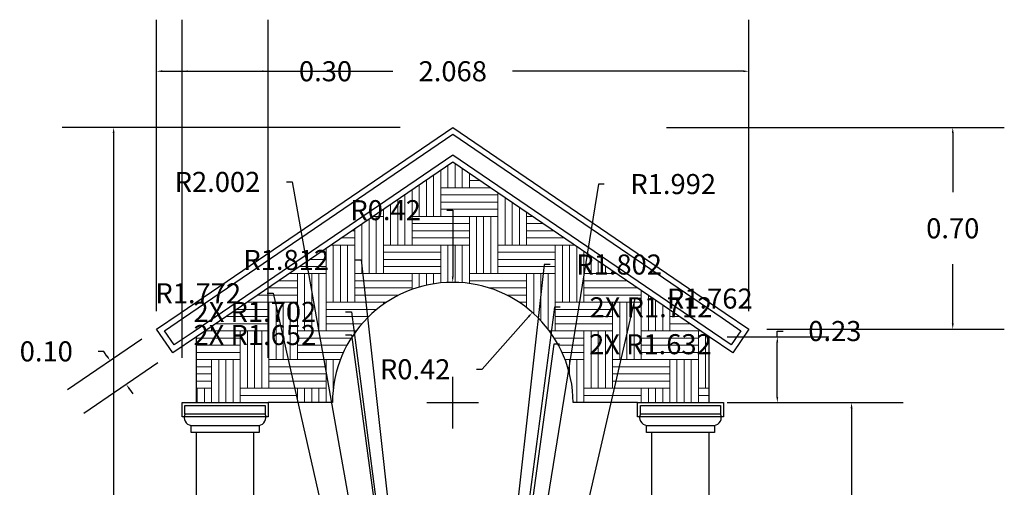
# Model space of a CAD drawing. Units: metres. Extents: x 10.71 to 14.27, y 9.22 to 13.79.
# Tile 2 of 2: x 10.83 to 14.27, y 12.15 to 13.79. Entities that reach past the tile are written whole.
import ezdxf

# ---------------------------------------------------------------- set-up
doc = ezdxf.new("R2010")
doc.units = ezdxf.units.M
doc.header["$MEASUREMENT"] = 0
for name, color, linetype, lineweight in [('A-ANNO-DIMS', 2, 'Continuous', 18), ('A-COLS', 7, 'Continuous', 30), ('A-ROOF', 7, 'Continuous', 30), ('A-ROOF-PATT', 252, 'Continuous', 13)]:
    doc.layers.add(name, color=color, linetype=linetype, lineweight=lineweight)
doc.styles.get("Standard").update_dxf_attribs({"font": 'arial.ttf'})
doc.dimstyles.get("Standard").update_dxf_attribs({"dimtxt": 0.07, "dimasz": 0.02, "dimexe": 0.18, "dimexo": 0.0625, "dimgap": 0.09, "dimtad": 0, "dimtih": 1, "dimtoh": 1, "dimzin": 0, "dimdsep": 46, "dimtxsty": 'Standard', "dimcen": 0.09, "dimadec": 0, "dimazin": 0, "dimtfac": 1, "dimtofl": 0, "dimtmove": 0, "dimatfit": 3, "dimfxl": 1, "dimfxlon": 1, "dimtolj": 1, "dimtzin": 0, "dimarcsym": 0})

# ---------------------------------------------------------------- blocks, each defined once
blk = doc.blocks.new('*D4')
at = {"layer": 'A-ANNO-DIMS', "color": 0, "lineweight": -2, "transparency": 16777216}
for p, q in [((12.1582, 13.4108), (10.9782, 13.4108)), ((11.1582, 13.3908), (11.1582, 11.7313)), ((11.1582, 9.8203), (11.1582, 11.4798)), ((11.1582, 9.8003), (10.9782, 9.8003))]:
    blk.add_line(p, q, dxfattribs=at)
at = {"layer": 'A-ANNO-DIMS', "color": 0, "transparency": 16777216}
for points in [[(11.1548, 13.3908), (11.1615, 13.3908), (11.1582, 13.4108)], [(11.1548, 9.8203), (11.1615, 9.8203), (11.1582, 9.8003)]]:
    blk.add_solid(points, dxfattribs=at)
at = {"layer": 'Defpoints', "color": 0, "transparency": 16777216}
for p in [(11.1582, 13.4108), (12.3422, 13.4108), (11.1842, 9.8003)]:
    blk.add_point(p, dxfattribs=at)
at = {"layer": 'A-ANNO-DIMS', "color": 0, "transparency": 16777216, "insert": (11.1582, 11.6055), "char_height": 0.07, "attachment_point": 5}
blk.add_mtext('\\A1;3.61', dxfattribs=at)
blk = doc.blocks.new('*D5')
at = {"layer": 'A-ANNO-DIMS', "color": 0, "lineweight": -2, "transparency": 16777216}
for p, q in [((13.4753, 12.6798), (13.4753, 12.6998)), ((13.4753, 12.6998), (13.4953, 12.6998)), ((13.2997, 12.6798), (13.6553, 12.6798)), ((13.4753, 12.4698), (13.4753, 12.6598)), ((13.2997, 12.4498), (13.6553, 12.4498))]:
    blk.add_line(p, q, dxfattribs=at)
at = {"layer": 'A-ANNO-DIMS', "color": 0, "transparency": 16777216}
for points in [[(13.472, 12.6598), (13.4786, 12.6598), (13.4753, 12.6798)], [(13.472, 12.4698), (13.4786, 12.4698), (13.4753, 12.4498)]]:
    blk.add_solid(points, dxfattribs=at)
at = {"layer": 'Defpoints', "color": 0, "transparency": 16777216}
for p in [(13.2372, 12.6798), (13.4753, 12.6798), (13.2372, 12.4498)]:
    blk.add_point(p, dxfattribs=at)
at = {"layer": 'A-ANNO-DIMS', "color": 0, "transparency": 16777216, "insert": (13.6762, 12.6998), "char_height": 0.07, "attachment_point": 5}
blk.add_mtext('\\A1;0.23', dxfattribs=at)
blk = doc.blocks.new('*D9')
at = {"layer": 'A-ANNO-DIMS', "color": 0, "lineweight": -2, "transparency": 16777216}
for p, q in [((12.445, 12.5663), (12.6068, 12.7498)), ((12.425, 12.5663), (12.445, 12.5663))]:
    blk.add_line(p, q, dxfattribs=at)
at = {"layer": 'A-ANNO-DIMS', "color": 0, "transparency": 16777216}
blk.add_solid([(12.6043, 12.752), (12.6093, 12.7476), (12.62, 12.7648)], dxfattribs=at)
at = {"layer": 'Defpoints', "color": 0, "transparency": 16777216}
for p in [(12.62, 12.7648), (12.3422, 12.4498)]:
    blk.add_point(p, dxfattribs=at)
at = {"layer": 'A-ANNO-DIMS', "color": 0, "transparency": 16777216, "insert": (12.2109, 12.5663), "char_height": 0.07, "attachment_point": 5}
blk.add_mtext('\\A1;R0.42', dxfattribs=at)
blk = doc.blocks.new('COL-ENTRANCE-CLASSICAL')
for p, q in [((0.1002, 1.975), (0.1002, 2.545)), ((0.3002, 1.975), (0.3002, 2.545)), ((0.1002, 0.1003), (0.1002, 1.8703)), ((0.3002, 0.1003), (0.3002, 1.8703)), ((0.1002, 0.1003), (0.3002, 0.1003))]:
    blk.add_line(p, q)
for points in [[(0.0502, 2.6498), (0.3502, 2.6498), (0.3502, 2.5998), (0.0502, 2.5998)], [(0.0602, 2.6398), (0.3402, 2.6398), (0.3402, 2.6098), (0.0602, 2.6098)], [(0.0816, 2.5705), (0.319, 2.5705), (0.319, 2.545), (0.0816, 2.545)], [(0.0502, 1.975), (0.3502, 1.975), (0.3502, 1.925), (0.0502, 1.925)], [(0.0602, 1.965), (0.3402, 1.965), (0.3402, 1.935), (0.0602, 1.935)], [(0.0816, 1.8957), (0.319, 1.8957), (0.319, 1.8703), (0.0816, 1.8703)], [(0.0502, 0.1003), (0.3502, 0.1003), (0.3502, 0.0503), (0.0502, 0.0503)], [(0.0602, 0.0903), (0.3402, 0.0903), (0.3402, 0.0603), (0.0602, 0.0603)], [(0.0002, 0.0503), (0.4002, 0.0503), (0.4002, 0.0003), (0.0002, 0.0003)], [(0.0102, 0.0403), (0.3902, 0.0403), (0.3902, 0.0103), (0.0102, 0.0103)]]:
    blk.add_lwpolyline(points, close=True)
for centre, radius, start, end in [((0.0856, 2.5981), 0.0279, 155.2605, 261.7776), ((0.3152, 2.5979), 0.0277, 277.9826, 25.4449), ((0.0856, 1.9233), 0.0279, 155.2605, 261.7776), ((0.3152, 1.9231), 0.0277, 277.9826, 25.4449)]:
    blk.add_arc(centre, radius, start, end)
blk = doc.blocks.new('*D15')
at = {"layer": 'A-ANNO-DIMS', "color": 0, "lineweight": -2, "transparency": 16777216}
for p, q in [((13.3997, 12.4498), (13.9146, 12.4498)), ((13.7346, 12.4298), (13.7346, 11.2512)), ((13.7346, 9.8203), (13.7346, 10.9988)), ((13.3997, 9.8003), (13.9146, 9.8003))]:
    blk.add_line(p, q, dxfattribs=at)
at = {"layer": 'A-ANNO-DIMS', "color": 0, "transparency": 16777216}
for points in [[(13.7313, 12.4298), (13.738, 12.4298), (13.7346, 12.4498)], [(13.7313, 9.8203), (13.738, 9.8203), (13.7346, 9.8003)]]:
    blk.add_solid(points, dxfattribs=at)
at = {"layer": 'Defpoints', "color": 0, "transparency": 16777216}
for p in [(13.3372, 12.4498), (13.7346, 12.4498), (13.3372, 9.8003)]:
    blk.add_point(p, dxfattribs=at)
at = {"layer": 'A-ANNO-DIMS', "color": 0, "transparency": 16777216, "insert": (13.7346, 11.125), "char_height": 0.07, "attachment_point": 5}
blk.add_mtext('\\A1;COLUMN 2.65 TYP.', dxfattribs=at)
blk = doc.blocks.new('*D19')
at = {"layer": 'A-ANNO-DIMS', "color": 0, "lineweight": -2, "transparency": 16777216}
for p, q in [((11.3082, 12.7686), (11.3082, 13.7868)), ((13.3762, 12.7686), (13.3762, 13.7868)), ((11.3283, 13.6068), (12.1334, 13.6068)), ((13.3562, 13.6068), (12.551, 13.6068))]:
    blk.add_line(p, q, dxfattribs=at)
at = {"layer": 'A-ANNO-DIMS', "color": 0, "transparency": 16777216}
for points in [[(11.3283, 13.6101), (11.3283, 13.6035), (11.3082, 13.6068)], [(13.3562, 13.6101), (13.3562, 13.6035), (13.3762, 13.6068)]]:
    blk.add_solid(points, dxfattribs=at)
at = {"layer": 'Defpoints', "color": 0, "transparency": 16777216}
for p in [(13.3762, 13.6068), (11.3082, 12.7061), (13.3762, 12.7061)]:
    blk.add_point(p, dxfattribs=at)
at = {"layer": 'A-ANNO-DIMS', "color": 0, "transparency": 16777216, "insert": (12.3422, 13.6068), "char_height": 0.07, "attachment_point": 5}
blk.add_mtext('\\A1;2.068', dxfattribs=at)
blk = doc.blocks.new('*D20')
at = {"layer": 'A-ANNO-DIMS', "color": 0, "lineweight": -2, "transparency": 16777216}
for p, q in [((13.0879, 13.4108), (14.2679, 13.4108)), ((14.0879, 13.3908), (14.0879, 13.1842)), ((14.0879, 12.7261), (14.0879, 12.9327)), ((13.4387, 12.7061), (14.2679, 12.7061))]:
    blk.add_line(p, q, dxfattribs=at)
at = {"layer": 'A-ANNO-DIMS', "color": 0, "transparency": 16777216}
for points in [[(14.0846, 13.3908), (14.0912, 13.3908), (14.0879, 13.4108)], [(14.0846, 12.7261), (14.0912, 12.7261), (14.0879, 12.7061)]]:
    blk.add_solid(points, dxfattribs=at)
at = {"layer": 'Defpoints', "color": 0, "transparency": 16777216}
for p in [(12.3422, 13.4108), (14.0879, 13.4108), (13.3762, 12.7061)]:
    blk.add_point(p, dxfattribs=at)
at = {"layer": 'A-ANNO-DIMS', "color": 0, "transparency": 16777216, "insert": (14.0879, 13.0584), "char_height": 0.07, "attachment_point": 5}
blk.add_mtext('\\A1;0.70', dxfattribs=at)
blk = doc.blocks.new('*D21')
at = {"layer": 'A-ANNO-DIMS', "color": 0, "lineweight": -2, "transparency": 16777216}
for p, q in [((11.2566, 12.6709), (10.9976, 12.4943)), ((11.1238, 12.6288), (11.1038, 12.6288)), ((11.135, 12.6122), (11.1238, 12.6288)), ((11.3129, 12.5883), (11.0539, 12.4117)), ((11.2139, 12.4965), (11.2251, 12.48))]:
    blk.add_line(p, q, dxfattribs=at)
at = {"layer": 'A-ANNO-DIMS', "color": 0, "transparency": 16777216}
for points in [[(11.1378, 12.6141), (11.1323, 12.6104), (11.1463, 12.5957)], [(11.2166, 12.4984), (11.2111, 12.4947), (11.2026, 12.5131)]]:
    blk.add_solid(points, dxfattribs=at)
at = {"layer": 'Defpoints', "color": 0, "transparency": 16777216}
for p in [(11.3082, 12.7061), (11.3646, 12.6235), (11.1463, 12.5957)]:
    blk.add_point(p, dxfattribs=at)
at = {"layer": 'A-ANNO-DIMS', "color": 0, "transparency": 16777216, "insert": (10.923, 12.6288), "char_height": 0.07, "attachment_point": 5}
blk.add_mtext('\\A1;0.10', dxfattribs=at)
blk = doc.blocks.new('*D24')
at = {"layer": 'A-ANNO-DIMS', "color": 0, "lineweight": -2, "transparency": 16777216}
for p, q in [((11.3972, 12.6068), (11.3972, 13.7868)), ((11.6972, 12.6068), (11.6972, 13.7868)), ((11.4172, 13.6068), (11.6772, 13.6068)), ((11.6972, 13.6068), (11.7172, 13.6068))]:
    blk.add_line(p, q, dxfattribs=at)
at = {"layer": 'A-ANNO-DIMS', "color": 0, "transparency": 16777216}
for points in [[(11.4172, 13.6101), (11.4172, 13.6035), (11.3972, 13.6068)], [(11.6772, 13.6101), (11.6772, 13.6035), (11.6972, 13.6068)]]:
    blk.add_solid(points, dxfattribs=at)
at = {"layer": 'Defpoints', "color": 0, "transparency": 16777216}
for p in [(11.6972, 13.6068), (11.3972, 11.775), (11.6972, 11.775)]:
    blk.add_point(p, dxfattribs=at)
at = {"layer": 'A-ANNO-DIMS', "color": 0, "transparency": 16777216, "insert": (11.898, 13.6068), "char_height": 0.07, "attachment_point": 5}
blk.add_mtext('\\A1;0.30', dxfattribs=at)
blk = doc.blocks.new('*D28')
at = {"layer": 'A-ANNO-DIMS', "color": 0, "lineweight": -2, "transparency": 16777216}
for p, q in [((11.762, 13.2204), (11.782, 13.2204)), ((11.782, 13.2204), (11.9886, 12.0574)), ((12.3422, 9.9765), (12.3422, 10.1565)), ((12.2522, 10.0665), (12.4322, 10.0665))]:
    blk.add_line(p, q, dxfattribs=at)
at = {"layer": 'A-ANNO-DIMS', "color": 0, "transparency": 16777216}
blk.add_solid([(11.9918, 12.058), (11.9853, 12.0568), (11.9921, 12.0377)], dxfattribs=at)
at = {"layer": 'Defpoints', "color": 0, "transparency": 16777216}
for p in [(11.9921, 12.0377), (12.3422, 10.0665)]:
    blk.add_point(p, dxfattribs=at)
at = {"layer": 'A-ANNO-DIMS', "color": 0, "transparency": 16777216, "insert": (11.5207, 13.2204), "char_height": 0.07, "attachment_point": 5}
blk.add_mtext('\\A1;R2.002', dxfattribs=at)
blk = doc.blocks.new('*D29')
at = {"layer": 'A-ANNO-DIMS', "color": 0, "lineweight": -2, "transparency": 16777216}
for p, q in [((12.8507, 13.2129), (12.6632, 12.0528)), ((12.8707, 13.2129), (12.8507, 13.2129)), ((12.3422, 9.9765), (12.3422, 10.1565)), ((12.2522, 10.0665), (12.4322, 10.0665))]:
    blk.add_line(p, q, dxfattribs=at)
at = {"layer": 'A-ANNO-DIMS', "color": 0, "transparency": 16777216}
blk.add_solid([(12.6599, 12.0533), (12.6665, 12.0522), (12.66, 12.033)], dxfattribs=at)
at = {"layer": 'Defpoints', "color": 0, "transparency": 16777216}
for p in [(12.66, 12.033), (12.3422, 10.0665)]:
    blk.add_point(p, dxfattribs=at)
at = {"layer": 'A-ANNO-DIMS', "color": 0, "transparency": 16777216, "insert": (13.1119, 13.2129), "char_height": 0.07, "attachment_point": 5}
blk.add_mtext('\\A1;R1.992', dxfattribs=at)
blk = doc.blocks.new('*D30')
at = {"layer": 'A-ANNO-DIMS', "color": 0, "lineweight": -2, "transparency": 16777216}
for p, q in [((12.002, 12.948), (12.022, 12.948)), ((12.022, 12.948), (12.1399, 11.8873)), ((12.3422, 9.9765), (12.3422, 10.1565)), ((12.2522, 10.0665), (12.4322, 10.0665))]:
    blk.add_line(p, q, dxfattribs=at)
at = {"layer": 'A-ANNO-DIMS', "color": 0, "transparency": 16777216}
blk.add_solid([(12.1432, 11.8877), (12.1365, 11.887), (12.1421, 11.8675)], dxfattribs=at)
at = {"layer": 'Defpoints', "color": 0, "transparency": 16777216}
for p in [(12.1421, 11.8675), (12.3422, 10.0665)]:
    blk.add_point(p, dxfattribs=at)
at = {"layer": 'A-ANNO-DIMS', "color": 0, "transparency": 16777216, "insert": (11.7607, 12.948), "char_height": 0.07, "attachment_point": 5}
blk.add_mtext('\\A1;R1.812', dxfattribs=at)
blk = doc.blocks.new('*D31')
at = {"layer": 'A-ANNO-DIMS', "color": 0, "lineweight": -2, "transparency": 16777216}
for p, q in [((12.6618, 12.932), (12.5442, 11.8773)), ((12.6818, 12.932), (12.6618, 12.932)), ((12.3422, 9.9765), (12.3422, 10.1565)), ((12.2522, 10.0665), (12.4322, 10.0665))]:
    blk.add_line(p, q, dxfattribs=at)
at = {"layer": 'A-ANNO-DIMS', "color": 0, "transparency": 16777216}
blk.add_solid([(12.5408, 11.8777), (12.5475, 11.8769), (12.5419, 11.8574)], dxfattribs=at)
at = {"layer": 'Defpoints', "color": 0, "transparency": 16777216}
for p in [(12.5419, 11.8574), (12.3422, 10.0665)]:
    blk.add_point(p, dxfattribs=at)
at = {"layer": 'A-ANNO-DIMS', "color": 0, "transparency": 16777216, "insert": (12.923, 12.932), "char_height": 0.07, "attachment_point": 5}
blk.add_mtext('\\A1;R1.802', dxfattribs=at)
blk = doc.blocks.new('*D32')
at = {"layer": 'A-ANNO-DIMS', "color": 0, "lineweight": -2, "transparency": 16777216}
for p, q in [((11.6948, 12.8315), (11.7148, 12.8315)), ((11.7148, 12.8315), (11.9457, 11.8141)), ((12.3422, 9.9765), (12.3422, 10.1565)), ((12.2522, 10.0665), (12.4322, 10.0665))]:
    blk.add_line(p, q, dxfattribs=at)
at = {"layer": 'A-ANNO-DIMS', "color": 0, "transparency": 16777216}
blk.add_solid([(11.9489, 11.8149), (11.9424, 11.8134), (11.9501, 11.7946)], dxfattribs=at)
at = {"layer": 'Defpoints', "color": 0, "transparency": 16777216}
for p in [(11.9501, 11.7946), (12.3422, 10.0665)]:
    blk.add_point(p, dxfattribs=at)
at = {"layer": 'A-ANNO-DIMS', "color": 0, "transparency": 16777216, "insert": (11.4536, 12.8315), "char_height": 0.07, "attachment_point": 5}
blk.add_mtext('\\A1;R1.772', dxfattribs=at)
blk = doc.blocks.new('*D33')
at = {"layer": 'A-ANNO-DIMS', "color": 0, "lineweight": -2, "transparency": 16777216}
for p, q in [((12.9783, 12.8131), (12.7443, 11.8026)), ((12.9983, 12.8131), (12.9783, 12.8131)), ((12.3422, 9.9765), (12.3422, 10.1565)), ((12.2522, 10.0665), (12.4322, 10.0665))]:
    blk.add_line(p, q, dxfattribs=at)
at = {"layer": 'A-ANNO-DIMS', "color": 0, "transparency": 16777216}
blk.add_solid([(12.7411, 11.8033), (12.7476, 11.8018), (12.7398, 11.7831)], dxfattribs=at)
at = {"layer": 'Defpoints', "color": 0, "transparency": 16777216}
for p in [(12.7398, 11.7831), (12.3422, 10.0665)]:
    blk.add_point(p, dxfattribs=at)
at = {"layer": 'A-ANNO-DIMS', "color": 0, "transparency": 16777216, "insert": (13.2396, 12.8131), "char_height": 0.07, "attachment_point": 5}
blk.add_mtext('\\A1;R1.762', dxfattribs=at)
blk = doc.blocks.new('*D34')
at = {"layer": 'A-ANNO-DIMS', "color": 0, "lineweight": -2, "transparency": 16777216}
for p, q in [((12.6971, 12.7827), (12.5666, 11.7839)), ((12.7171, 12.7827), (12.6971, 12.7827)), ((12.3422, 9.9765), (12.3422, 10.1565)), ((12.2522, 10.0665), (12.4322, 10.0665))]:
    blk.add_line(p, q, dxfattribs=at)
at = {"layer": 'A-ANNO-DIMS', "color": 0, "transparency": 16777216}
blk.add_solid([(12.5633, 11.7844), (12.5699, 11.7835), (12.564, 11.7641)], dxfattribs=at)
at = {"layer": 'Defpoints', "color": 0, "transparency": 16777216}
for p in [(12.564, 11.7641), (12.3422, 10.0665)]:
    blk.add_point(p, dxfattribs=at)
at = {"layer": 'A-ANNO-DIMS', "color": 0, "transparency": 16777216, "insert": (13.0341, 12.7827), "char_height": 0.07, "attachment_point": 5}
blk.add_mtext('\\A1;2X R1.712', dxfattribs=at)
blk = doc.blocks.new('*D35')
at = {"layer": 'A-ANNO-DIMS', "color": 0, "lineweight": -2, "transparency": 16777216}
for p, q in [((11.9683, 12.7667), (11.9883, 12.7667)), ((11.9883, 12.7667), (12.1184, 11.7739)), ((12.3422, 9.9765), (12.3422, 10.1565)), ((12.2522, 10.0665), (12.4322, 10.0665))]:
    blk.add_line(p, q, dxfattribs=at)
at = {"layer": 'A-ANNO-DIMS', "color": 0, "transparency": 16777216}
blk.add_solid([(12.1217, 11.7744), (12.1151, 11.7735), (12.121, 11.7541)], dxfattribs=at)
at = {"layer": 'Defpoints', "color": 0, "transparency": 16777216}
for p in [(12.121, 11.7541), (12.3422, 10.0665)]:
    blk.add_point(p, dxfattribs=at)
at = {"layer": 'A-ANNO-DIMS', "color": 0, "transparency": 16777216, "insert": (11.6512, 12.7667), "char_height": 0.07, "attachment_point": 5}
blk.add_mtext('\\A1;2X R1.702', dxfattribs=at)
blk = doc.blocks.new('*D36')
at = {"layer": 'A-ANNO-DIMS', "color": 0, "lineweight": -2, "transparency": 16777216}
for p, q in [((11.9683, 12.686), (11.9883, 12.686)), ((11.9883, 12.686), (12.1184, 11.7235)), ((12.3422, 9.9765), (12.3422, 10.1565)), ((12.2522, 10.0665), (12.4322, 10.0665))]:
    blk.add_line(p, q, dxfattribs=at)
at = {"layer": 'A-ANNO-DIMS', "color": 0, "transparency": 16777216}
blk.add_solid([(12.1217, 11.7239), (12.1151, 11.723), (12.121, 11.7037)], dxfattribs=at)
at = {"layer": 'Defpoints', "color": 0, "transparency": 16777216}
for p in [(12.121, 11.7037), (12.3422, 10.0665)]:
    blk.add_point(p, dxfattribs=at)
at = {"layer": 'A-ANNO-DIMS', "color": 0, "transparency": 16777216, "insert": (11.6513, 12.686), "char_height": 0.07, "attachment_point": 5}
blk.add_mtext('\\A1;2X R1.652', dxfattribs=at)
blk = doc.blocks.new('*D37')
at = {"layer": 'A-ANNO-DIMS', "color": 0, "lineweight": -2, "transparency": 16777216}
for p, q in [((12.6954, 12.6538), (12.5656, 11.7034)), ((12.7154, 12.6538), (12.6954, 12.6538)), ((12.3422, 9.9765), (12.3422, 10.1565)), ((12.2522, 10.0665), (12.4322, 10.0665))]:
    blk.add_line(p, q, dxfattribs=at)
at = {"layer": 'A-ANNO-DIMS', "color": 0, "transparency": 16777216}
blk.add_solid([(12.5623, 11.7038), (12.5689, 11.7029), (12.5629, 11.6835)], dxfattribs=at)
at = {"layer": 'Defpoints', "color": 0, "transparency": 16777216}
for p in [(12.5629, 11.6835), (12.3422, 10.0665)]:
    blk.add_point(p, dxfattribs=at)
at = {"layer": 'A-ANNO-DIMS', "color": 0, "transparency": 16777216, "insert": (13.0324, 12.6538), "char_height": 0.07, "attachment_point": 5}
blk.add_mtext('\\A1;2X R1.632', dxfattribs=at)
blk = doc.blocks.new('*D38')
at = {"layer": 'A-ANNO-DIMS', "color": 0, "lineweight": -2, "transparency": 16777216}
for p, q in [((12.3219, 13.1218), (12.3419, 13.1218)), ((12.3419, 13.1218), (12.342, 12.8898)), ((12.3422, 12.3598), (12.3422, 12.5398)), ((12.2522, 12.4498), (12.4322, 12.4498))]:
    blk.add_line(p, q, dxfattribs=at)
at = {"layer": 'A-ANNO-DIMS', "color": 0, "transparency": 16777216}
blk.add_solid([(12.3453, 12.8898), (12.3387, 12.8898), (12.342, 12.8698)], dxfattribs=at)
at = {"layer": 'Defpoints', "color": 0, "transparency": 16777216}
for p in [(12.342, 12.8698), (12.3422, 12.4498)]:
    blk.add_point(p, dxfattribs=at)
at = {"layer": 'A-ANNO-DIMS', "color": 0, "transparency": 16777216, "insert": (12.1078, 13.1218), "char_height": 0.07, "attachment_point": 5}
blk.add_mtext('\\A1;R0.42', dxfattribs=at)

msp = doc.modelspace()

# ---------------------------------------------------------------- hatches: boundary and pattern name
at = {"layer": 'A-ROOF-PATT'}
h = msp.add_hatch(dxfattribs=at)
h.set_pattern_fill('µØ°Å4', color=256, scale=0.2)
h.set_pattern_definition([(0, (0, 0), (0.1, 0.1), [0.2, -0.2]), (0, (0, 0.025), (0.1, 0.1), [0.2, -0.2]), (0, (0, 0.05), (0.1, 0.1), [0.2, -0.2]), (0, (0, 0.075), (0.1, 0.1), [0.2, -0.2]), (0, (0, 0.1), (0.1, 0.1), [0.1, -0.3]), (90, (0, 0.1), (0.1, 0.1), [0.2, -0.2]), (90, (0.025, 0.1), (0.1, 0.1), [0.2, -0.2]), (90, (0.05, 0.1), (0.1, 0.1), [0.2, -0.2]), (90, (0.075, 0.1), (0.1, 0.1), [0.2, -0.2]), (90, (0.1, 0.1), (0.1, 0.1), [0.1, -0.3])])
h.paths.add_polyline_path([(12.3422, 13.2898), (11.4472, 12.6798), (11.4472, 12.4498), (11.6972, 12.4498), (11.9222, 12.4498, -1), (12.7622, 12.4498), (12.9872, 12.4498), (13.2372, 12.4498), (13.2372, 12.6798)])

# ---------------------------------------------------------------- linework, layer by layer
at = {"layer": 'A-ROOF'}
for p, q in [((11.4472, 12.4498), (11.4472, 12.6798)), ((13.2372, 12.4498), (13.2372, 12.6798)), ((11.9222, 12.4498), (11.6972, 12.4498)), ((12.9872, 12.4498), (12.7622, 12.4498))]:
    msp.add_line(p, q, dxfattribs=at)
for points in [[(11.3082, 12.7061), (11.3909, 12.7624), (12.3422, 13.4108), (13.2935, 12.7624), (13.3762, 12.7061), (13.3198, 12.6235), (13.2372, 12.6798), (12.3422, 13.2898), (11.4472, 12.6798), (11.3646, 12.6235)], [(11.336, 12.7008), (11.4021, 12.7459), (12.3422, 13.3866), (13.2823, 12.7459), (13.3484, 12.7008), (13.3146, 12.6512), (13.2485, 12.6963), (12.3422, 13.314), (11.4359, 12.6963), (11.3698, 12.6512)]]:
    msp.add_lwpolyline(points, close=True, dxfattribs=at)
msp.add_arc((12.3422, 12.4498), 0.42, 0, 180, dxfattribs=at)

# ---------------------------------------------------------------- block references
at = {"layer": 'A-COLS'}
for p in [(11.347, 9.8), (12.937, 9.8)]:
    msp.add_blockref('COL-ENTRANCE-CLASSICAL', p, dxfattribs=at)

# ---------------------------------------------------------------- dimensions: what is measured, and where the dimension line sits
at = {"layer": 'A-ANNO-DIMS'}
for base, p1, p2, override, picture, middle in [((13.3762, 13.6068), (11.3082, 12.7061), (13.3762, 12.7061), {"dimdec": 3, "dimlfac": 1, "dimrnd": 0, "dimzin": 0, "dimdsep": 46, "dimlunit": 2}, '*D19', (12.3422, 13.6068)), ((11.6972, 13.6068), (11.3972, 11.775), (11.6972, 11.775), {"dimdec": 2, "dimlfac": 1, "dimrnd": 0, "dimzin": 0, "dimdsep": 46, "dimlunit": 2}, '*D24', (11.898, 13.6068))]:
    dim = msp.add_linear_dim(base=base, p1=p1, p2=p2, dimstyle='Standard', override=override, dxfattribs=at)
    dim.commit()
    dim.dimension.update_dxf_attribs({"geometry": picture, "text_midpoint": middle})
for base, p1, p2, angle, override, picture, middle in [((11.1582, 13.4108), (11.1842, 9.8003), (12.3422, 13.4108), 90, {"dimclrd": 0, "dimclre": 0, "dimclrt": 0}, '*D4', (11.1582, 11.6055)), ((14.0879, 13.4108), (13.3762, 12.7061), (12.3422, 13.4108), 90, {"dimdec": 2, "dimlfac": 1, "dimrnd": 0, "dimzin": 0, "dimdsep": 46, "dimlunit": 2}, '*D20', (14.0879, 13.0584)), ((13.4753, 12.6798), (13.2372, 12.4498), (13.2372, 12.6798), 90, {"dimclrd": 0, "dimclre": 0, "dimclrt": 0}, '*D5', (13.6762, 12.6998)), ((11.1463, 12.5957), (11.3646, 12.6235), (11.3082, 12.7061), 124.2769, {"dimdec": 2, "dimlfac": 1, "dimrnd": 0, "dimzin": 0, "dimdsep": 46, "dimlunit": 2}, '*D21', (10.923, 12.6288))]:
    dim = msp.add_linear_dim(base=base, p1=p1, p2=p2, angle=angle, dimstyle='Standard', override=override, dxfattribs=at)
    dim.commit()
    dim.dimension.update_dxf_attribs({"geometry": picture, "text_midpoint": middle})
for center, mpoint, override, picture, middle in [((12.3422, 10.0665), (11.9921, 12.0377), {"dimdec": 3, "dimlfac": 1, "dimrnd": 0, "dimzin": 0, "dimdsep": 46, "dimlunit": 2}, '*D28', (11.5207, 13.2204)), ((12.3422, 10.0665), (12.66, 12.033), {"dimdec": 3, "dimlfac": 1, "dimrnd": 0, "dimzin": 0, "dimdsep": 46, "dimlunit": 2}, '*D29', (13.1119, 13.2129)), ((12.3422, 12.4498), (12.342, 12.8698), {"dimdec": 2, "dimlfac": 1, "dimrnd": 0, "dimzin": 0, "dimdsep": 46, "dimlunit": 2}, '*D38', (12.1078, 13.1218)), ((12.3422, 10.0665), (12.1421, 11.8675), {"dimdec": 3, "dimlfac": 1, "dimrnd": 0, "dimzin": 0, "dimdsep": 46, "dimlunit": 2}, '*D30', (11.7607, 12.948)), ((12.3422, 10.0665), (12.5419, 11.8574), {"dimdec": 3, "dimlfac": 1, "dimrnd": 0, "dimzin": 0, "dimdsep": 46, "dimlunit": 2}, '*D31', (12.923, 12.932)), ((12.3422, 10.0665), (11.9501, 11.7946), {"dimdec": 3, "dimlfac": 1, "dimrnd": 0, "dimzin": 0, "dimdsep": 46, "dimlunit": 2}, '*D32', (11.4536, 12.8315)), ((12.3422, 10.0665), (12.7398, 11.7831), {"dimdec": 3, "dimlfac": 1, "dimrnd": 0, "dimzin": 0, "dimdsep": 46, "dimlunit": 2}, '*D33', (13.2396, 12.8131)), ((12.3422, 12.4498), (12.62, 12.7648), {"dimclrd": 0, "dimclre": 0, "dimclrt": 0}, '*D9', (12.2109, 12.5663))]:
    dim = msp.add_radius_dim(center=center, mpoint=mpoint, dimstyle='Standard', override=override, dxfattribs=at)
    dim.commit()
    dim.dimension.update_dxf_attribs({"geometry": picture, "text_midpoint": middle, "dimtype": 164})
for mpoint, picture, middle in [((12.121, 11.7541), '*D35', (11.6512, 12.7667)), ((12.564, 11.7641), '*D34', (13.0341, 12.7827)), ((12.121, 11.7037), '*D36', (11.6513, 12.686)), ((12.5629, 11.6835), '*D37', (13.0324, 12.6538))]:
    dim = msp.add_radius_dim(center=(12.3422, 10.0665), mpoint=mpoint, text='2X <>', dimstyle='Standard', override={"dimdec": 3, "dimlfac": 1, "dimrnd": 0, "dimzin": 0, "dimdsep": 46, "dimlunit": 2}, dxfattribs=at)
    dim.commit()
    dim.dimension.update_dxf_attribs({"geometry": picture, "text_midpoint": middle, "dimtype": 164})
dim = msp.add_linear_dim(base=(13.7346, 12.4498), p1=(13.3372, 9.8003), p2=(13.3372, 12.4498), angle=90, text='COLUMN <> TYP.', dimstyle='Standard', override={"dimdec": 2, "dimlfac": 1, "dimrnd": 0, "dimzin": 0, "dimdsep": 46, "dimlunit": 2}, dxfattribs=at)
dim.commit()
dim.dimension.update_dxf_attribs({"geometry": '*D15', "text_midpoint": (13.7346, 11.125)})

doc.saveas('drawing.dxf')
